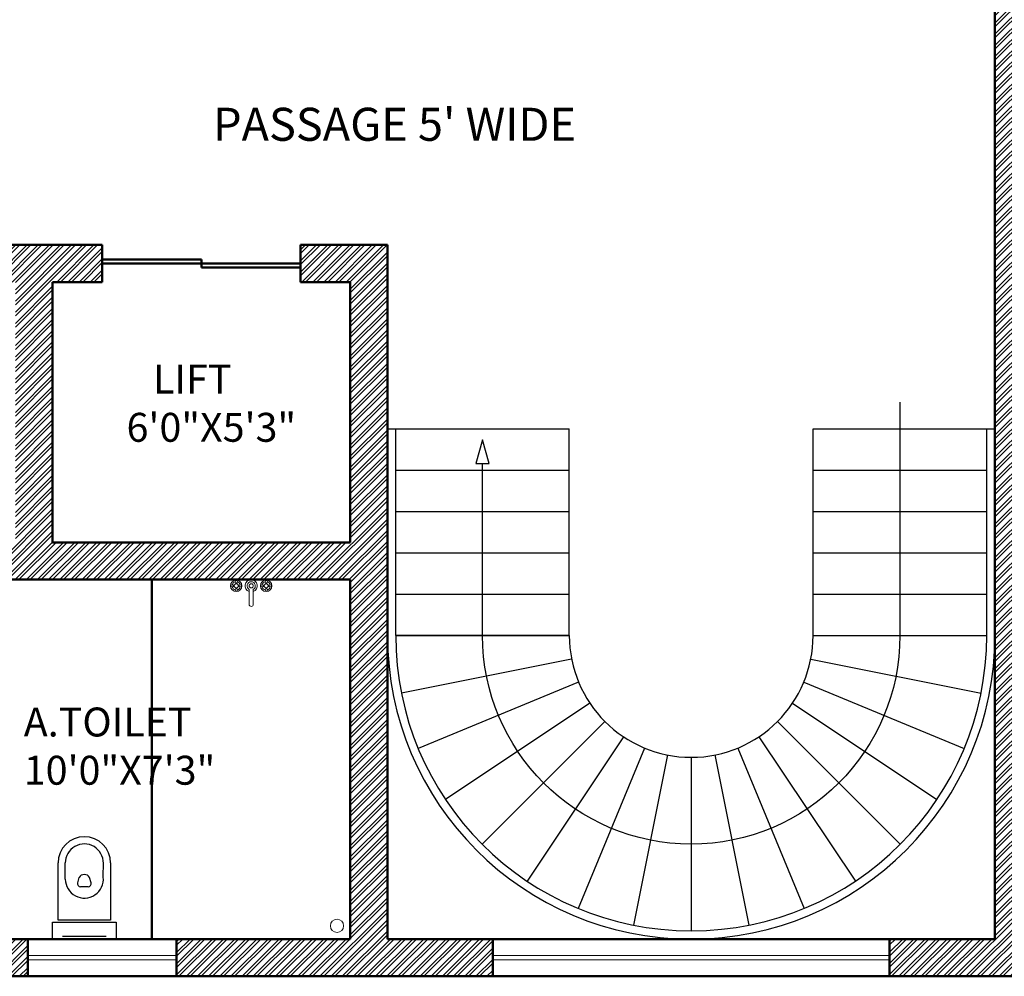
# Model space of a CAD drawing. Units: inches. Extents: x 3590 to 5167, y 65 to 1917.
# Tile 28 of 100: x 4688 to 4927, y 1326 to 1558. Entities that reach past the tile are written whole.
import ezdxf

# ---------------------------------------------------------------- set-up
doc = ezdxf.new("R2010")
doc.units = ezdxf.units.IN
for name, color, linetype, lineweight in [('A-AREA-IDEN', 7, 'Continuous', 18), ('A-FLOR-FIXT', 8, 'Continuous', 18), ('A-FLOR-STRS', 7, 'Continuous', 25), ('A-GLAZ', 4, 'Continuous', 18), ('A-WALL', 7, 'Continuous', 50), ('A-WALL-PATT', 251, 'Continuous', 13)]:
    doc.layers.add(name, color=color, linetype=linetype, lineweight=lineweight)
doc.layers.add('SANTEH', color=7, linetype='Continuous')
doc.styles.get("Standard").update_dxf_attribs({"font": 'arial.ttf'})

# ---------------------------------------------------------------- blocks, each defined once
blk = doc.blocks.new('*U99')
blk.add_line((-21, 0), (21, 0))
blk = doc.blocks.new('*U100')
at = {"layer": 'A-FLOR-STRS', "color": 0, "linetype": 'ByBlock', "lineweight": -2, "transparency": 16777216}
for p, rotation in [((4076.01, 1459), 89.99999999999982), ((4066.16, 1458.03), 101.2499999999998), ((4085.86, 1458.03), 78.7499999999998), ((4056.69, 1455.15), 112.4999999999998), ((4095.34, 1455.15), 67.4999999999998), ((4047.96, 1450.49), 123.7499999999997), ((4104.07, 1450.49), 56.24999999999984), ((4040.3, 1444.21), 134.9999999999996), ((4111.72, 1444.21), 44.99999999999992), ((4034.02, 1436.56), 146.2499999999996), ((4118, 1436.56), 33.74999999999991), ((4029.36, 1427.82), 157.4999999999995), ((4122.67, 1427.82), 22.49999999999996), ((4026.48, 1418.35), 168.7499999999995), ((4125.54, 1418.35), 11.25), ((4025.51, 1408.5), 180)]:
    blk.add_blockref('*U99', p, dxfattribs=dict(at, rotation=rotation))
blk.add_blockref('*U99', (4126.51, 1408.5), dxfattribs=at)
blk = doc.blocks.new('y3')
at = {"layer": 'SANTEH', "ltscale": 5}
for p, q in [((37.5, 130.7), (37.5, 520.7)), ((87.5, 410.7), (87.5, 520.7)), ((346.6, 426.1), (347.5, 520.7)), ((397.5, 520.7), (397.5, 130.7)), ((171.9, 384.5), (181.1, 421.3)), ((263.1, 384.5), (253.9, 421.3)), ((244.3, 357.8), (190.7, 357.8)), ((397.5, 130.7), (37.5, 130.7)), ((67.5, 20.7), (367.5, 20.7))]:
    blk.add_line(p, q, dxfattribs=at)
blk.add_lwpolyline([(0, 115), (435, 115), (435, 0), (0, 0), (0, 115)], dxfattribs=at)
for centre, radius, start, end in [((217.5, 520.7), 180, 0, 180), ((217.5, 520.7), 130, 359.15795, 180), ((217.5, 410.7), 130, 180, 5.98548), ((217.5, 399.9), 42.2, 30.52342, 149.47658), ((190.7, 377.8), 20, 160.50385, 270), ((244.3, 377.8), 20, 270, 19.49615)]:
    blk.add_arc(centre, radius, start, end, dxfattribs=at)
blk = doc.blocks.new('Faucet - Bathroom top')
for p, q in [((-4.107, 0.125), (-4.375, 0.125)), ((-3.75, 0.4788), (-3.75, 0.75)), ((-3.5, 0.482), (-3.5, 0.75)), ((-3.1461, 0.125), (-2.875, 0.125)), ((3.143, 0.125), (2.875, 0.125)), ((3.5, 0.4788), (3.5, 0.75)), ((3.75, 0.482), (3.75, 0.75)), ((4.1039, 0.125), (4.375, 0.125)), ((-4.1039, -0.125), (-4.375, -0.125)), ((-3.75, -0.4821), (-3.75, -0.75)), ((-3.5, -0.4789), (-3.5, -0.75)), ((-3.143, -0.125), (-2.875, -0.125)), ((-0.5, -0.8639), (-0.5, -4.5)), ((0.5, -4.5), (0.5, -0.8631)), ((3.1461, -0.125), (2.875, -0.125)), ((3.5, -0.4821), (3.5, -0.75)), ((3.75, -0.4789), (3.75, -0.75)), ((4.107, -0.125), (4.375, -0.125))]:
    blk.add_line(p, q)
for centre, radius in [((-3.625, 0), 1.375), ((-4.625, 0), 0.2795), ((-3.625, 0), 0.5), ((-3.625, 1), 0.2795), ((-2.625, 0), 0.2795), ((0, 0), 0.5), ((3.625, 0), 1.375), ((2.625, 0), 0.2795), ((3.625, 0), 0.5), ((3.625, 1), 0.2795), ((4.625, 0), 0.2795), ((-3.625, -1), 0.2795), ((3.625, -1), 0.2795)]:
    blk.add_circle(centre, radius)
for centre, radius, start, end in [((-3.625, 0), 1, 105.2407, 164.2093), ((-3.625, 0), 1, 16.44125, 74.07887), ((0, 0), 1.5, 289.6514, 250.3603), ((0, 0), 1, 300.3431, 239.7554), ((3.625, 0), 1, 106.12, 164.0884), ((3.625, 0), 1, 16.23422, 73.90469), ((-3.625, 0), 1, 196.2342, 253.9047), ((-3.625, 0), 1, 286.12, 344.0884), ((3.625, 0), 1, 196.4413, 254.0789), ((3.625, 0), 1, 285.2407, 344.2093), ((0, -4.5), 0.5, 180, 0)]:
    blk.add_arc(centre, radius, start, end)

msp = doc.modelspace()

# ---------------------------------------------------------------- hatches: boundary and pattern name
at = {"layer": 'A-WALL-PATT', "transparency": 33554687}
h = msp.add_hatch(dxfattribs=at)
h.set_pattern_fill('ANSI32', color=256, scale=0.2)
h.paths.add_polyline_path([(4684.27, 1806), (4591.27, 1806), (4591.27, 1797), (4639.27, 1797), (4639.27, 1791), (4648.27, 1791), (4648.27, 1797), (4684.27, 1797)])
h.paths.add_polyline_path([(4543.27, 1806), (4420.27, 1806), (4420.27, 1785), (4429.27, 1785), (4429.27, 1797), (4445.92, 1797), (4543.27, 1797)])
h.paths.add_polyline_path([(4828.27, 1806), (4744.27, 1806), (4744.27, 1797), (4828.27, 1797)])
h.paths.add_polyline_path([(4648.27, 1755), (4639.27, 1755), (4639.27, 1656), (4546.27, 1656), (4546.27, 1650), (4549.27, 1650), (4549.27, 1554), (4429.27, 1554), (4429.27, 1584), (4420.27, 1584), (4420.27, 1539), (4429.27, 1539), (4429.27, 1545), (4639.27, 1545), (4639.27, 1539), (4648.27, 1539), (4648.27, 1560), (4639.27, 1560), (4639.27, 1554), (4555.27, 1554), (4555.27, 1650), (4639.27, 1650), (4639.27, 1590), (4648.27, 1590)])
h.paths.add_polyline_path([(4516.27, 1656), (4429.27, 1656), (4429.27, 1737), (4420.27, 1737), (4420.27, 1620), (4429.27, 1620), (4429.27, 1650), (4516.27, 1650)], flags=17)
h.paths.add_polyline_path([(5080.27, 1806), (4888.27, 1806), (4888.27, 1797), (4924.27, 1797), (4924.27, 1755), (4933.27, 1755), (4933.27, 1797), (5071.27, 1797), (5071.27, 1335), (4933.27, 1335), (4933.27, 1566), (4924.27, 1566), (4924.27, 1335), (4898.77, 1335), (4898.77, 1326), (5080.27, 1326)])
h.paths.add_polyline_path([(4933.27, 1719), (4924.27, 1719), (4924.27, 1638), (4933.27, 1638)], flags=17)
h.paths.add_polyline_path([(4802.77, 1335), (4777.27, 1335), (4777.27, 1503), (4756.27, 1503), (4756.27, 1494), (4768.27, 1494), (4768.27, 1431), (4696.27, 1431), (4696.27, 1494), (4708.27, 1494), (4708.27, 1503), (4639.27, 1503), (4639.27, 1494), (4687.27, 1494), (4687.27, 1431), (4681.27, 1431), (4681.27, 1422), (4768.27, 1422), (4768.27, 1335), (4726.27, 1335), (4726.27, 1326), (4802.77, 1326)])
h.paths.add_polyline_path([(4690.27, 1335), (4648.27, 1335), (4648.27, 1352.87), (4648.27, 1422), (4651.27, 1422), (4651.27, 1431), (4639.27, 1431), (4639.27, 1335), (4633.27, 1335), (4633.27, 1326), (4690.27, 1326)])
h.paths.add_polyline_path([(4585.27, 1335), (4584.72, 1335), (4429.27, 1335), (4429.27, 1491), (4420.27, 1491), (4420.27, 1326), (4585.27, 1326)])

# ---------------------------------------------------------------- linework, layer by layer
at = {"layer": 'A-FLOR-FIXT'}
msp.add_circle((4765.07, 1338.21), 1.6, dxfattribs=at)
at = {"layer": 'A-FLOR-STRS'}
for p, q in [((4777.27, 1458.5), (4821.27, 1458.5)), ((4779.27, 1408.5), (4779.27, 1458.5)), ((4821.27, 1408.5), (4821.27, 1458.5)), ((4880.27, 1458.5), (4924.27, 1458.5)), ((4880.27, 1408.5), (4880.27, 1458.5)), ((4922.27, 1408.5), (4922.27, 1458.5)), ((4779.27, 1448.5), (4821.27, 1448.5)), ((4880.27, 1448.5), (4922.27, 1448.5)), ((4779.27, 1438.5), (4821.27, 1438.5)), ((4880.27, 1438.5), (4922.27, 1438.5)), ((4779.27, 1428.5), (4821.27, 1428.5)), ((4880.27, 1428.5), (4922.27, 1428.5)), ((4779.27, 1418.5), (4821.27, 1418.5)), ((4880.27, 1418.5), (4922.27, 1418.5)), ((4779.27, 1408.5), (4821.27, 1408.5))]:
    msp.add_line(p, q, dxfattribs=at)
msp.add_lwpolyline([(4901.27, 1464.94), (4901.27, 1408.5, -1), (4800.27, 1408.5), (4800.27, 1450.11)], format="xyb", dxfattribs=at)
msp.add_lwpolyline([(4800.27, 1455.87), (4798.64, 1450.11), (4801.91, 1450.11)], close=True, dxfattribs=at)
for radius in [73.5, 71.5, 29.5]:
    msp.add_arc((4850.77, 1408.5), radius, 180, 0, dxfattribs=at)
at = {"layer": 'A-GLAZ'}
for p, q in [((4726.27, 1331), (4690.27, 1331)), ((4726.27, 1330), (4690.27, 1330)), ((4898.77, 1331), (4802.77, 1331)), ((4898.77, 1330), (4802.77, 1330))]:
    msp.add_line(p, q, dxfattribs=at)
at = {"layer": 'A-WALL'}
for p, q in [((4924.27, 1335), (4924.27, 1719)), ((4708.27, 1503), (4639.27, 1503)), ((4708.27, 1494), (4708.27, 1503)), ((4777.27, 1503), (4756.27, 1503)), ((4756.27, 1494), (4756.27, 1503)), ((4777.27, 1335), (4777.27, 1503)), ((4708.27, 1499.5), (4732.27, 1499.5)), ((4708.27, 1498.5), (4756.27, 1498.5)), ((4732.27, 1499.5), (4732.27, 1497.5)), ((4732.27, 1497.5), (4756.27, 1497.5)), ((4708.27, 1494), (4696.27, 1494)), ((4696.27, 1431), (4696.27, 1494)), ((4768.27, 1494), (4756.27, 1494)), ((4768.27, 1431), (4768.27, 1494)), ((4768.27, 1431), (4696.27, 1431)), ((4768.27, 1422), (4681.27, 1422)), ((4720.27, 1335), (4720.27, 1422)), ((4768.27, 1335), (4768.27, 1422)), ((4768.27, 1335), (4648.27, 1335)), ((4690.27, 1335), (4690.27, 1326)), ((4726.27, 1335), (4726.27, 1326)), ((4924.27, 1335), (4777.27, 1335)), ((4802.77, 1335), (4802.77, 1326)), ((4898.77, 1335), (4898.77, 1326))]:
    msp.add_line(p, q, dxfattribs=at)
msp.add_lwpolyline([(5080.27, 1806), (5080.27, 1326), (4420.27, 1326), (4420.27, 1806)], close=True, dxfattribs=at)

# ---------------------------------------------------------------- block references
at = {"layer": 'A-FLOR-FIXT'}
msp.add_blockref('Faucet - Bathroom top', (4744.31, 1420.5), dxfattribs=at)
at = {"layer": 'A-FLOR-FIXT', "xscale": 0.0353848906415677, "yscale": 0.0353848906415677, "zscale": 0.0353848906415677}
msp.add_blockref('y3', (4696.24, 1335), dxfattribs=at)
at = {"layer": 'A-FLOR-STRS', "xscale": -1, "rotation": 180}
msp.add_blockref('*U100', (774.76, 2817), dxfattribs=at)

# ---------------------------------------------------------------- texts
at = {"layer": 'A-AREA-IDEN', "attachment_point": 1}
for s, width, insert, char_height in [("{\\fTimes New Roman|b0|i0|c0|p18;PASSAGE 5' WIDE}", 131.4857, (4735.07, 1536.2), 8), ('{\\fTimes New Roman|b0|i0|c0|p18;   LIFT\\P6\'0"X5\'3"}', 67.3508, (4714.15, 1474.03), 7), ('{\\fTimes New Roman|b0|i0|c0|p18;A.TOILET\\P10\'0"X7\'3"}', 67.3508, (4689.28, 1391.04), 7)]:
    msp.add_mtext_dynamic_manual_height_columns(s, width=width, gutter_width=12.5, heights=[0], dxfattribs=dict(at, insert=insert, char_height=char_height))

doc.saveas('drawing.dxf')
